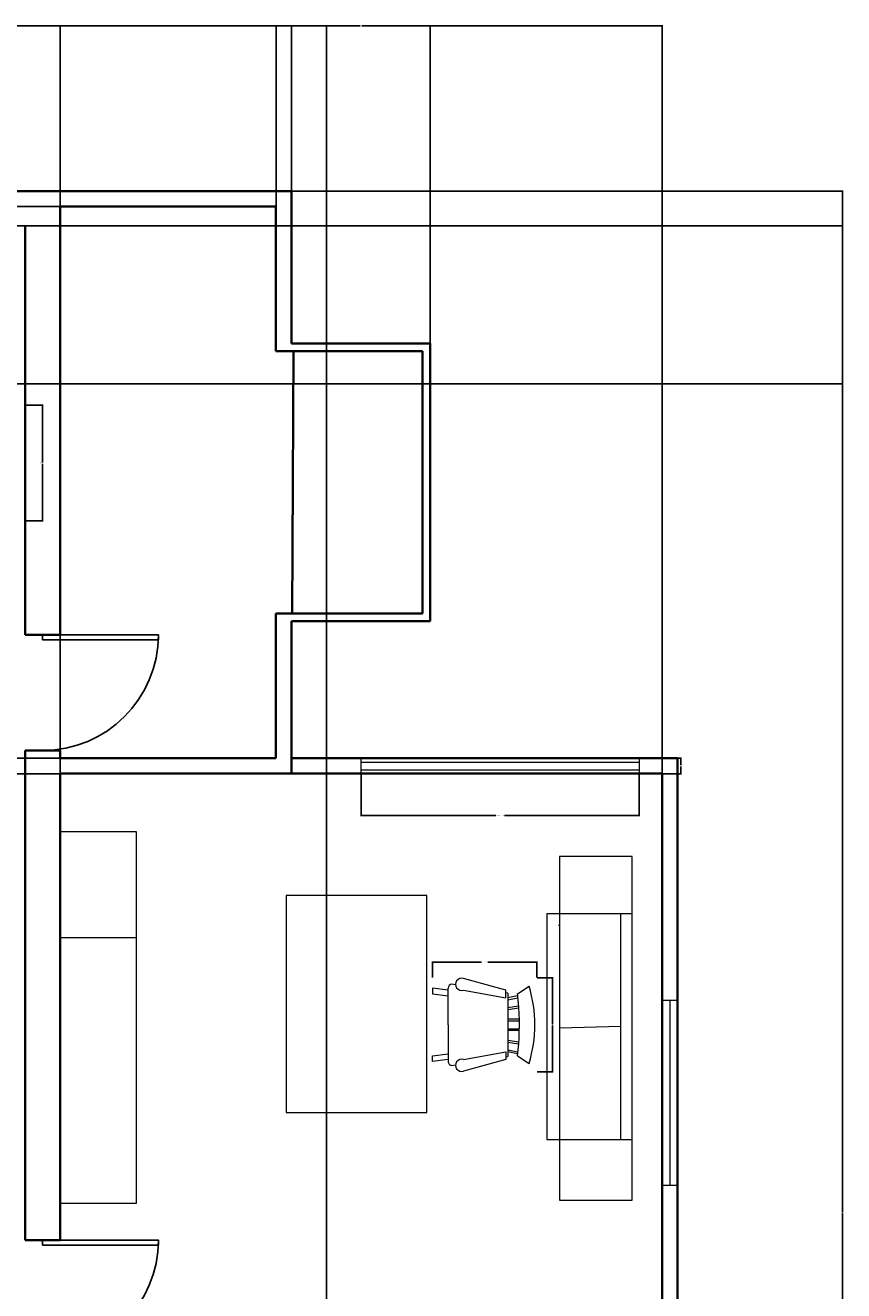
# Model space of a CAD drawing. Units: inches. Extents: x 2024 to 2965, y 1692 to 2308.
# Tile 8 of 8: x 2753 to 2965, y 1980 to 2308. Entities that reach past the tile are written whole.
import ezdxf

# ---------------------------------------------------------------- set-up
doc = ezdxf.new("R2010")
doc.units = ezdxf.units.IN
for name, color, linetype, lineweight in [('A-ANNO-DIMS', 2, 'Continuous', 18), ('A-DOOR', 3, 'Continuous', 25), ('A-FLOR-CASE', 33, 'Continuous', 20), ('A-FURN', 8, 'Continuous', 18), ('A-GLAZ', 4, 'Continuous', 18), ('A-WALL', 7, 'Continuous', 35)]:
    doc.layers.add(name, color=color, linetype=linetype, lineweight=lineweight)
doc.styles.get("Standard").update_dxf_attribs({"font": 'arial.ttf'})
doc.dimstyles.get("Standard").update_dxf_attribs({"dimtxt": 0.18, "dimasz": 0.18, "dimexe": 0.18, "dimexo": 0.0625, "dimgap": 0.09, "dimtad": 0, "dimtih": 1, "dimtoh": 1, "dimdec": 4, "dimzin": 0, "dimdsep": 46, "dimtxsty": 'Standard', "dimcen": 0.09, "dimadec": 0, "dimazin": 0, "dimtfac": 1, "dimtdec": 4, "dimtofl": 0, "dimtmove": 0, "dimatfit": 3, "dimfxl": 1, "dimtolj": 1, "dimtzin": 0, "dimarcsym": 0})

# ---------------------------------------------------------------- blocks, each defined once
blk = doc.blocks.new('*U7')
for p, q in [((0, 0), (0, -6)), ((40, 0), (40, -6))]:
    blk.add_line(p, q)
blk.add_lwpolyline([(0, 0), (0, 40), (1.75, 40), (1.75, 0)], close=True)
blk.add_arc((0, 0), 40, 0, 90)
blk = doc.blocks.new('Chair - Rocking')
for p, q in [((-8, -4.5), (-10, -1.5)), ((8, -4.5), (10, -1.5)), ((-7.5, -4.5), (-7, -7)), ((-6.5, -7), (-7.02225, -4.43)), ((-4.5, -7), (-4.96674, -4.19951)), ((-4, -7), (-4.40532, -4.16272)), ((-1.5, -4.05012), (-1.5, -7)), ((-1, -7), (-1, -4.05012)), ((1, -7), (1, -4.04655)), ((1.5, -4.05012), (1.5, -7)), ((4, -7), (4.40187, -4.18694)), ((4.5, -7), (4.96761, -4.19437)), ((6.5, -7), (7, -4.4057)), ((7.5, -4.5), (7, -7)), ((-9, -7.5), (-12, -18.49999)), ((-7, -7.5), (-9, -7.5)), ((-9, -18.49999), (-7, -7.5)), ((-8.23428, -6.99939), (-8.3093, -7.47958)), ((-8.23041, -7), (8.23915, -7)), ((7, -7.5), (9, -7.5)), ((9, -18.49999), (7, -7.5)), ((8.31071, -7.48854), (8.23449, -7.00073)), ((9, -7.5), (12, -18.49999)), ((-10.36644, -20.64523), (-10.5, -21.49999)), ((-9, -22.49999), (-9.5, -26.49999)), ((0, -22.49999), (-9.5, -22.49999)), ((-8, -26.49999), (-7.5, -22.49999)), ((0, -22.49999), (9.5, -22.49999)), ((8, -26.49999), (7.5, -22.49999)), ((9, -22.49999), (9.5, -26.49999)), ((10.5, -21.49999), (10.3575, -20.58798)), ((-9.5, -26.49999), (-8, -26.49999)), ((9.5, -26.49999), (8, -26.49999))]:
    blk.add_line(p, q)
for centre, radius, start, end in [((0, -34.08333), 34.08333, 72.93847, 107.0615), ((0, -68.25004), 64.25, 93.92211, 97.15267), ((0, -68.25004), 64.25, 82.84733, 93.92211), ((-10.5, -18.99999), 1.58114, 161.5651, 18.43495), ((10.5, -18.99999), 1.58114, 161.5651, 18.43495), ((-9.5, -21.49999), 1, 180, 270), ((9.5, -21.49999), 1, 270, 0)]:
    blk.add_arc(centre, radius, start, end)
blk = doc.blocks.new('WIN-72-D4')
for p, q in [((0, 3), (72, 3)), ((0, 1), (72, 1))]:
    blk.add_line(p, q)
for points in [[(0, 0), (0, 4)], [(72, 4), (72, 0)]]:
    blk.add_lwpolyline(points)
blk = doc.blocks.new('*D35')
at = {"layer": 'A-ANNO-DIMS', "color": 0, "lineweight": -2, "transparency": 16777216}
for p, q in [((2840.03, 2113.71), (2840.03, 2102.79)), ((2912.03, 2113.71), (2912.03, 2102.79)), ((2840.21, 2102.97), (2874.91, 2102.97)), ((2911.85, 2102.97), (2877.15, 2102.97))]:
    blk.add_line(p, q, dxfattribs=at)
at = {"layer": 'A-ANNO-DIMS', "color": 0, "transparency": 16777216}
for points in [[(2840.21, 2103), (2840.21, 2102.94), (2840.03, 2102.97)], [(2911.85, 2103), (2911.85, 2102.94), (2912.03, 2102.97)]]:
    blk.add_solid(points, dxfattribs=at)
at = {"layer": 'Defpoints', "color": 0, "transparency": 16777216}
for p in [(2840.03, 2113.77), (2912.03, 2113.77), (2912.03, 2102.97)]:
    blk.add_point(p, dxfattribs=at)
at = {"layer": 'A-ANNO-DIMS', "color": 0, "transparency": 16777216, "insert": (2876.03, 2102.97), "char_height": 0.18, "attachment_point": 5}
blk.add_mtext('\\A1;WINDOW 72 TYP.', dxfattribs=at)
blk = doc.blocks.new('*D36')
at = {"layer": 'A-ANNO-DIMS', "color": 0, "lineweight": -2, "transparency": 16777216}
for p, q in [((2912.09, 2117.77), (2923.01, 2117.77)), ((2922.83, 2117.59), (2922.83, 2115.95)), ((2922.83, 2113.95), (2922.83, 2115.59)), ((2912.09, 2113.77), (2923.01, 2113.77))]:
    blk.add_line(p, q, dxfattribs=at)
at = {"layer": 'A-ANNO-DIMS', "color": 0, "transparency": 16777216}
for points in [[(2922.8, 2117.59), (2922.86, 2117.59), (2922.83, 2117.77)], [(2922.8, 2113.95), (2922.86, 2113.95), (2922.83, 2113.77)]]:
    blk.add_solid(points, dxfattribs=at)
at = {"layer": 'Defpoints', "color": 0, "transparency": 16777216}
for p in [(2912.03, 2117.77), (2922.83, 2117.77), (2912.03, 2113.77)]:
    blk.add_point(p, dxfattribs=at)
at = {"layer": 'A-ANNO-DIMS', "color": 0, "transparency": 16777216, "insert": (2922.83, 2115.77), "char_height": 0.18, "attachment_point": 5}
blk.add_mtext('\\A1;4 TYP.', dxfattribs=at)
blk = doc.blocks.new('*D53')
at = {"layer": 'A-ANNO-DIMS', "color": 0, "lineweight": -2, "transparency": 16777216}
for p, q in [((2858.52, 2060.96), (2858.52, 2065.13)), ((2858.7, 2064.95), (2871.23, 2064.95)), ((2885.34, 2064.95), (2872.8, 2064.95)), ((2885.52, 2060.96), (2885.52, 2065.13))]:
    blk.add_line(p, q, dxfattribs=at)
at = {"layer": 'A-ANNO-DIMS', "color": 0, "transparency": 16777216}
for points in [[(2858.7, 2064.98), (2858.7, 2064.92), (2858.52, 2064.95)], [(2885.34, 2064.98), (2885.34, 2064.92), (2885.52, 2064.95)]]:
    blk.add_solid(points, dxfattribs=at)
at = {"layer": 'Defpoints', "color": 0, "transparency": 16777216}
for p in [(2885.52, 2064.95), (2858.52, 2060.9), (2885.52, 2060.9)]:
    blk.add_point(p, dxfattribs=at)
at = {"layer": 'A-ANNO-DIMS', "color": 0, "transparency": 16777216, "insert": (2872.02, 2064.95), "char_height": 0.18, "attachment_point": 5}
blk.add_mtext('\\A1;ROCKER 27', dxfattribs=at)
blk = doc.blocks.new('*D54')
at = {"layer": 'A-ANNO-DIMS', "color": 0, "lineweight": -2, "transparency": 16777216}
for p, q in [((2885.58, 2060.9), (2889.75, 2060.9)), ((2889.57, 2060.72), (2889.57, 2048.86)), ((2889.57, 2036.64), (2889.57, 2048.5)), ((2885.58, 2036.46), (2889.75, 2036.46))]:
    blk.add_line(p, q, dxfattribs=at)
at = {"layer": 'A-ANNO-DIMS', "color": 0, "transparency": 16777216}
for points in [[(2889.54, 2060.72), (2889.6, 2060.72), (2889.57, 2060.9)], [(2889.54, 2036.64), (2889.6, 2036.64), (2889.57, 2036.46)]]:
    blk.add_solid(points, dxfattribs=at)
at = {"layer": 'Defpoints', "color": 0, "transparency": 16777216}
for p in [(2885.52, 2060.9), (2885.52, 2036.46), (2889.57, 2036.46)]:
    blk.add_point(p, dxfattribs=at)
at = {"layer": 'A-ANNO-DIMS', "color": 0, "transparency": 16777216, "insert": (2889.57, 2048.68), "char_height": 0.18, "attachment_point": 5}
blk.add_mtext('\\A1;24', dxfattribs=at)
blk = doc.blocks.new('*D71')
at = {"layer": 'A-ANNO-DIMS', "color": 0, "lineweight": -2, "transparency": 16777216}
for p, q in [((2752.94, 2209.27), (2757.56, 2209.27)), ((2757.38, 2209.09), (2757.38, 2194.46)), ((2757.38, 2179.45), (2757.38, 2194.09)), ((2752.94, 2179.27), (2757.56, 2179.27))]:
    blk.add_line(p, q, dxfattribs=at)
at = {"layer": 'A-ANNO-DIMS', "color": 0, "transparency": 16777216}
for points in [[(2757.35, 2209.09), (2757.41, 2209.09), (2757.38, 2209.27)], [(2757.35, 2179.45), (2757.41, 2179.45), (2757.38, 2179.27)]]:
    blk.add_solid(points, dxfattribs=at)
at = {"layer": 'Defpoints', "color": 0, "transparency": 16777216}
for p in [(2752.88, 2209.27), (2752.88, 2179.27), (2757.38, 2179.27)]:
    blk.add_point(p, dxfattribs=at)
at = {"layer": 'A-ANNO-DIMS', "color": 0, "transparency": 16777216, "insert": (2757.38, 2194.27), "char_height": 0.18, "attachment_point": 5}
blk.add_mtext('\\A1;RANGE 30', dxfattribs=at)
blk = doc.blocks.new('*D76')
at = {"layer": 'A-ANNO-DIMS', "color": 0, "lineweight": -2, "transparency": 16777216}
for p, q in [((2718.97, 2264.77), (2964.97, 2264.77)), ((2964.79, 2264.59), (2964.79, 2000.12)), ((2964.79, 1735.28), (2964.79, 1999.75)), ((2515.28, 1735.1), (2964.97, 1735.1))]:
    blk.add_line(p, q, dxfattribs=at)
at = {"layer": 'A-ANNO-DIMS', "color": 0, "transparency": 16777216}
for points in [[(2964.76, 2264.59), (2964.82, 2264.59), (2964.79, 2264.77)], [(2964.76, 1735.28), (2964.82, 1735.28), (2964.79, 1735.1)]]:
    blk.add_solid(points, dxfattribs=at)
at = {"layer": 'Defpoints', "color": 0, "transparency": 16777216}
for p in [(2718.91, 2264.77), (2515.22, 1735.1), (2964.79, 1735.1)]:
    blk.add_point(p, dxfattribs=at)
at = {"layer": 'A-ANNO-DIMS', "color": 0, "transparency": 16777216, "insert": (2964.79, 1999.94), "char_height": 0.18, "attachment_point": 5}
blk.add_mtext('\\A1;529.7', dxfattribs=at)
blk = doc.blocks.new('*D87')
at = {"layer": 'A-ANNO-DIMS', "color": 0, "lineweight": -2, "transparency": 16777216}
for p, q in [((2761.91, 2260.84), (2761.91, 2307.73)), ((2762.09, 2307.55), (2789.69, 2307.55)), ((2817.73, 2307.55), (2790.12, 2307.55)), ((2817.91, 2260.84), (2817.91, 2307.73))]:
    blk.add_line(p, q, dxfattribs=at)
at = {"layer": 'A-ANNO-DIMS', "color": 0, "transparency": 16777216}
for points in [[(2762.09, 2307.58), (2762.09, 2307.52), (2761.91, 2307.55)], [(2817.73, 2307.58), (2817.73, 2307.52), (2817.91, 2307.55)]]:
    blk.add_solid(points, dxfattribs=at)
at = {"layer": 'Defpoints', "color": 0, "transparency": 16777216}
for p in [(2817.91, 2307.55), (2761.91, 2260.77), (2817.91, 2260.77)]:
    blk.add_point(p, dxfattribs=at)
at = {"layer": 'A-ANNO-DIMS', "color": 0, "transparency": 16777216, "insert": (2789.91, 2307.55), "char_height": 0.18, "attachment_point": 5}
blk.add_mtext('\\A1;56', dxfattribs=at)
blk = doc.blocks.new('*D88')
at = {"layer": 'A-ANNO-DIMS', "color": 0, "lineweight": -2, "transparency": 16777216}
for p, q in [((2817.84, 2260.77), (2024.5, 2260.77)), ((2024.68, 2260.59), (2024.68, 2189.46)), ((2024.68, 2117.95), (2024.68, 2189.09)), ((2817.84, 2117.77), (2024.5, 2117.77))]:
    blk.add_line(p, q, dxfattribs=at)
at = {"layer": 'A-ANNO-DIMS', "color": 0, "transparency": 16777216}
for points in [[(2024.65, 2260.59), (2024.71, 2260.59), (2024.68, 2260.77)], [(2024.65, 2117.95), (2024.71, 2117.95), (2024.68, 2117.77)]]:
    blk.add_solid(points, dxfattribs=at)
at = {"layer": 'Defpoints', "color": 0, "transparency": 16777216}
for p in [(2817.91, 2260.77), (2024.68, 2117.77), (2817.91, 2117.77)]:
    blk.add_point(p, dxfattribs=at)
at = {"layer": 'A-ANNO-DIMS', "color": 0, "transparency": 16777216, "insert": (2024.68, 2189.27), "char_height": 0.18, "attachment_point": 5}
blk.add_mtext('\\A1;143', dxfattribs=at)
blk = doc.blocks.new('*D89')
at = {"layer": 'A-ANNO-DIMS', "color": 0, "lineweight": -2, "transparency": 16777216}
for p, q in [((2821.91, 2225.34), (2821.91, 2307.73)), ((2822.09, 2307.55), (2839.69, 2307.55)), ((2857.73, 2307.55), (2840.12, 2307.55)), ((2857.91, 2225.34), (2857.91, 2307.73))]:
    blk.add_line(p, q, dxfattribs=at)
at = {"layer": 'A-ANNO-DIMS', "color": 0, "transparency": 16777216}
for points in [[(2822.09, 2307.58), (2822.09, 2307.52), (2821.91, 2307.55)], [(2857.73, 2307.58), (2857.73, 2307.52), (2857.91, 2307.55)]]:
    blk.add_solid(points, dxfattribs=at)
at = {"layer": 'Defpoints', "color": 0, "transparency": 16777216}
for p in [(2857.91, 2307.55), (2821.91, 2225.27), (2857.91, 2225.27)]:
    blk.add_point(p, dxfattribs=at)
at = {"layer": 'A-ANNO-DIMS', "color": 0, "transparency": 16777216, "insert": (2839.91, 2307.55), "char_height": 0.18, "attachment_point": 5}
blk.add_mtext('\\A1;36', dxfattribs=at)
blk = doc.blocks.new('*D99')
at = {"layer": 'A-ANNO-DIMS', "color": 0, "lineweight": -2, "transparency": 16777216}
for p, q in [((2668.91, 1952.85), (2668.91, 2307.73)), ((2669.09, 2307.55), (2749.48, 2307.55)), ((2830.78, 2307.55), (2750.39, 2307.55)), ((2830.96, 1952.97), (2830.96, 2307.73))]:
    blk.add_line(p, q, dxfattribs=at)
at = {"layer": 'A-ANNO-DIMS', "color": 0, "transparency": 16777216}
for points in [[(2669.09, 2307.58), (2669.09, 2307.52), (2668.91, 2307.55)], [(2830.78, 2307.58), (2830.78, 2307.52), (2830.96, 2307.55)]]:
    blk.add_solid(points, dxfattribs=at)
at = {"layer": 'Defpoints', "color": 0, "transparency": 16777216}
for p in [(2830.96, 2307.55), (2668.91, 1952.79), (2830.96, 1952.91)]:
    blk.add_point(p, dxfattribs=at)
at = {"layer": 'A-ANNO-DIMS', "color": 0, "transparency": 16777216, "insert": (2749.93, 2307.55), "char_height": 0.18, "attachment_point": 5}
blk.add_mtext('\\A1;162.06', dxfattribs=at)
blk = doc.blocks.new('*D100')
at = {"layer": 'A-ANNO-DIMS', "color": 0, "lineweight": -2, "transparency": 16777216}
for p, q in [((2761.91, 2113.84), (2761.91, 2307.73)), ((2762.09, 2307.55), (2839.59, 2307.55)), ((2917.84, 2307.55), (2840.33, 2307.55)), ((2918.02, 2113.84), (2918.02, 2307.73))]:
    blk.add_line(p, q, dxfattribs=at)
at = {"layer": 'A-ANNO-DIMS', "color": 0, "transparency": 16777216}
for points in [[(2762.09, 2307.58), (2762.09, 2307.52), (2761.91, 2307.55)], [(2917.84, 2307.58), (2917.84, 2307.52), (2918.02, 2307.55)]]:
    blk.add_solid(points, dxfattribs=at)
at = {"layer": 'Defpoints', "color": 0, "transparency": 16777216}
for p in [(2918.02, 2307.55), (2761.91, 2113.77), (2918.02, 2113.77)]:
    blk.add_point(p, dxfattribs=at)
at = {"layer": 'A-ANNO-DIMS', "color": 0, "transparency": 16777216, "insert": (2839.96, 2307.55), "char_height": 0.18, "attachment_point": 5}
blk.add_mtext('\\A1;156.1', dxfattribs=at)
blk = doc.blocks.new('*D101')
at = {"layer": 'A-ANNO-DIMS', "color": 0, "lineweight": -2, "transparency": 16777216}
for p, q in [((2917.96, 2113.77), (2024.5, 2113.77)), ((2024.68, 2113.59), (2024.68, 2035.52)), ((2024.68, 1957.09), (2024.68, 2035.16)), ((2917.96, 1956.91), (2024.5, 1956.91))]:
    blk.add_line(p, q, dxfattribs=at)
at = {"layer": 'A-ANNO-DIMS', "color": 0, "transparency": 16777216}
for points in [[(2024.65, 2113.59), (2024.71, 2113.59), (2024.68, 2113.77)], [(2024.65, 1957.09), (2024.71, 1957.09), (2024.68, 1956.91)]]:
    blk.add_solid(points, dxfattribs=at)
at = {"layer": 'Defpoints', "color": 0, "transparency": 16777216}
for p in [(2024.68, 2113.77), (2918.02, 2113.77), (2918.02, 1956.91)]:
    blk.add_point(p, dxfattribs=at)
at = {"layer": 'A-ANNO-DIMS', "color": 0, "transparency": 16777216, "insert": (2024.68, 2035.34), "char_height": 0.18, "attachment_point": 5}
blk.add_mtext('\\A1;156.87', dxfattribs=at)
blk = doc.blocks.new('*D108')
at = {"layer": 'A-ANNO-DIMS', "color": 0, "lineweight": -2, "transparency": 16777216}
for p, q in [((2542.97, 2255.77), (2964.97, 2255.77)), ((2964.79, 2255.59), (2964.79, 2235.45)), ((2964.79, 2214.95), (2964.79, 2235.09)), ((2542.97, 2214.77), (2964.97, 2214.77))]:
    blk.add_line(p, q, dxfattribs=at)
at = {"layer": 'A-ANNO-DIMS', "color": 0, "transparency": 16777216}
for points in [[(2964.76, 2255.59), (2964.82, 2255.59), (2964.79, 2255.77)], [(2964.76, 2214.95), (2964.82, 2214.95), (2964.79, 2214.77)]]:
    blk.add_solid(points, dxfattribs=at)
at = {"layer": 'Defpoints', "color": 0, "transparency": 16777216}
for p in [(2542.91, 2255.77), (2542.91, 2214.77), (2964.79, 2214.77)]:
    blk.add_point(p, dxfattribs=at)
at = {"layer": 'A-ANNO-DIMS', "color": 0, "transparency": 16777216, "insert": (2964.79, 2235.27), "char_height": 0.18, "attachment_point": 5}
blk.add_mtext('\\A1;41', dxfattribs=at)

msp = doc.modelspace()

# ---------------------------------------------------------------- linework, layer by layer
at = {"layer": 'A-FLOR-CASE'}
msp.add_line((2761.9061, 2071.3419), (2781.6533, 2071.3419), dxfattribs=at)
msp.add_lwpolyline([(2761.9061, 2098.7975), (2781.6533, 2098.7975), (2781.6533, 2002.3743), (2761.9061, 2002.3743)], close=True, dxfattribs=at)
at = {"layer": 'A-FURN'}
msp.add_line((2907.2786, 2048.2115), (2891.3771, 2047.7868), dxfattribs=at)
for points in [[(2910.2786, 2092.2967), (2891.3771, 2092.2967), (2891.3771, 2003.2768), (2910.2786, 2003.2768)], [(2856.9964, 2082.1743), (2820.5529, 2082.1743), (2820.5529, 2025.9368), (2856.9964, 2025.9368)], [(2910.2786, 2077.4284), (2888.1413, 2077.4284), (2888.1413, 2018.9946), (2910.2786, 2018.9946)]]:
    msp.add_lwpolyline(points, close=True, dxfattribs=at)
for points in [[(2907.2786, 2018.9946), (2907.2786, 2077.4284)], [(2891.3771, 2074.4284), (2891.1413, 2074.4284)]]:
    msp.add_lwpolyline(points, dxfattribs=at)
at = {"layer": 'A-GLAZ'}
for p, q in [((2918.0192, 2055.0483), (2918.0192, 2007.0483)), ((2920.0192, 2055.0483), (2920.0192, 2007.0483))]:
    msp.add_line(p, q, dxfattribs=at)
for points in [[(2918.0192, 2055.0483), (2922.0192, 2055.0483)], [(2922.0192, 2007.0483), (2918.0192, 2007.0483)]]:
    msp.add_lwpolyline(points, dxfattribs=at)
at = {"layer": 'A-WALL'}
for p, q in [((2161.9061, 2264.7736), (2821.9061, 2264.7736)), ((2821.9061, 2264.7736), (2821.9061, 2225.2736)), ((2761.9061, 2260.7736), (2761.9061, 2149.7736)), ((2761.9061, 2260.7736), (2817.9061, 2260.7736)), ((2817.9061, 2260.7736), (2817.9061, 2223.2736)), ((2752.9061, 2255.7736), (2752.9061, 2149.7736)), ((2821.9061, 2225.2736), (2857.9061, 2225.2736)), ((2857.9061, 2225.2736), (2857.9061, 2153.2736)), ((2817.9061, 2223.2736), (2855.9061, 2223.2736)), ((2822.4663, 2223.2736), (2822.0994, 2155.2736)), ((2855.9061, 2223.2736), (2855.9061, 2155.2736)), ((2817.9061, 2155.2736), (2855.9061, 2155.2736)), ((2817.9061, 2155.2736), (2817.9061, 2117.7736)), ((2821.9061, 2153.2736), (2857.9061, 2153.2736)), ((2821.9061, 2153.2736), (2821.9061, 2113.7736)), ((2752.9061, 2149.7736), (2761.9061, 2149.7736)), ((2752.9061, 2119.7736), (2761.9061, 2119.7736)), ((2752.9061, 2119.7736), (2752.9061, 1992.9082)), ((2761.9061, 2117.7736), (2817.9061, 2117.7736)), ((2821.9061, 2117.7736), (2918.0192, 2117.7736)), ((2918.0192, 2117.7736), (2922.0192, 2117.7736)), ((2922.0192, 2117.7736), (2922.0192, 1952.9082)), ((2761.9061, 2113.7736), (2821.9061, 2113.7736)), ((2821.9061, 2113.7736), (2918.0192, 2113.7736)), ((2918.0192, 2113.7736), (2918.0192, 1956.9082)), ((2761.9061, 1992.9082), (2752.9061, 1992.9082))]:
    msp.add_line(p, q, dxfattribs=at)
for points in [[(2761.9061, 2119.7736), (2761.9061, 2117.7736)], [(2821.9061, 2119.7736), (2821.9061, 2113.7736)], [(2761.9061, 2113.7736), (2761.9061, 1992.9082)]]:
    msp.add_lwpolyline(points, dxfattribs=at)

# ---------------------------------------------------------------- block references
at = {"layer": 'A-DOOR', "xscale": 0.75, "yscale": 0.75, "zscale": 0.75, "rotation": 270}
for p in [(2757.4061, 2149.7736), (2757.4061, 1992.9082)]:
    msp.add_blockref('*U7', p, dxfattribs=at)
at = {"layer": 'A-FURN', "rotation": 270}
msp.add_blockref('Chair - Rocking', (2885.0177, 2048.6777), dxfattribs=at)
at = {"layer": 'A-GLAZ'}
msp.add_blockref('WIN-72-D4', (2840.0321, 2113.774), dxfattribs=at)

# ---------------------------------------------------------------- dimensions: what is measured, and where the dimension line sits
at = {"layer": 'A-ANNO-DIMS'}
for base, p1, p2, override, picture, middle in [((2830.9627, 2307.5486), (2668.9061, 1952.7881), (2830.9627, 1952.9082), {"dimdec": 2, "dimlfac": 1, "dimrnd": 0, "dimzin": 0, "dimdsep": 46, "dimlunit": 2}, '*D99', (2749.9344, 2307.5486)), ((2817.9061, 2307.5486), (2761.9061, 2260.7736), (2817.9061, 2260.7736), {"dimdec": 0, "dimlfac": 1, "dimrnd": 0, "dimzin": 0, "dimdsep": 46, "dimlunit": 2}, '*D87', (2789.9061, 2307.5486)), ((2918.0192, 2307.5486), (2761.9061, 2113.7736), (2918.0192, 2113.7736), {"dimdec": 1, "dimlfac": 1, "dimrnd": 0, "dimzin": 0, "dimdsep": 46, "dimlunit": 2}, '*D100', (2839.9627, 2307.5486)), ((2857.9061, 2307.5486), (2821.9061, 2225.2736), (2857.9061, 2225.2736), {"dimdec": 0, "dimlfac": 1, "dimrnd": 0, "dimzin": 0, "dimdsep": 46, "dimlunit": 2}, '*D89', (2839.9061, 2307.5486))]:
    dim = msp.add_linear_dim(base=base, p1=p1, p2=p2, dimstyle='Standard', override=override, dxfattribs=at)
    dim.commit()
    dim.dimension.update_dxf_attribs({"geometry": picture, "text_midpoint": middle})
for base, p1, p2, angle, override, picture, middle in [((2964.7942, 1735.0986), (2718.9061, 2264.7736), (2515.2195, 1735.0986), 90, {"dimdec": 1, "dimlfac": 1, "dimrnd": 0, "dimzin": 0, "dimdsep": 46, "dimlunit": 2}, '*D76', (2964.7942, 1999.9361)), ((2024.6844, 2117.7736), (2817.9061, 2260.7736), (2817.9061, 2117.7736), 90, {"dimdec": 0, "dimlfac": 1, "dimrnd": 0, "dimzin": 0, "dimdsep": 46, "dimlunit": 2}, '*D88', (2024.6844, 2189.2736)), ((2964.7942, 2214.7696), (2542.9061, 2255.7736), (2542.9061, 2214.7696), 90, {"dimdec": 0, "dimlfac": 1, "dimrnd": 0, "dimzin": 0, "dimdsep": 46, "dimlunit": 2}, '*D108', (2964.7942, 2235.2716)), ((2024.6844, 2113.7736), (2918.0192, 1956.9082), (2918.0192, 2113.7736), 90, {"dimdec": 2, "dimlfac": 1, "dimrnd": 0, "dimzin": 0, "dimdsep": 46, "dimlunit": 2}, '*D101', (2024.6844, 2035.3409)), ((2889.5676, 2036.4602), (2885.5177, 2060.8953), (2885.5177, 2036.4602), 270, {"dimdec": 0, "dimlfac": 1, "dimrnd": 0, "dimzin": 0, "dimdsep": 46, "dimlunit": 2}, '*D54', (2889.5676, 2048.6777))]:
    dim = msp.add_linear_dim(base=base, p1=p1, p2=p2, angle=angle, dimstyle='Standard', override=override, dxfattribs=at)
    dim.commit()
    dim.dimension.update_dxf_attribs({"geometry": picture, "text_midpoint": middle})
for base, p1, p2, angle, text, picture, middle in [((2757.3769, 2179.2724), (2752.8769, 2209.2724), (2752.8769, 2179.2724), 270, 'RANGE <>', '*D71', (2757.3769, 2194.2724)), ((2922.8317, 2117.7736), (2912.0317, 2113.7736), (2912.0317, 2117.7736), 90, '<> TYP.', '*D36', (2922.8317, 2115.7736))]:
    dim = msp.add_linear_dim(base=base, p1=p1, p2=p2, angle=angle, text=text, dimstyle='Standard', override={"dimdec": 0, "dimlfac": 1, "dimrnd": 0, "dimzin": 0, "dimdsep": 46, "dimlunit": 2}, dxfattribs=at)
    dim.commit()
    dim.dimension.update_dxf_attribs({"geometry": picture, "text_midpoint": middle})
for base, p1, p2, text, picture, middle in [((2912.0317, 2102.9736), (2840.0317, 2113.7736), (2912.0317, 2113.7736), 'WINDOW <> TYP.', '*D35', (2876.0317, 2102.9736)), ((2885.5177, 2064.9453), (2858.5177, 2060.8953), (2885.5177, 2060.8953), 'ROCKER <>', '*D53', (2872.0177, 2064.9453))]:
    dim = msp.add_linear_dim(base=base, p1=p1, p2=p2, text=text, dimstyle='Standard', override={"dimdec": 0, "dimlfac": 1, "dimrnd": 0, "dimzin": 0, "dimdsep": 46, "dimlunit": 2}, dxfattribs=at)
    dim.commit()
    dim.dimension.update_dxf_attribs({"geometry": picture, "text_midpoint": middle})

doc.saveas('drawing.dxf')
